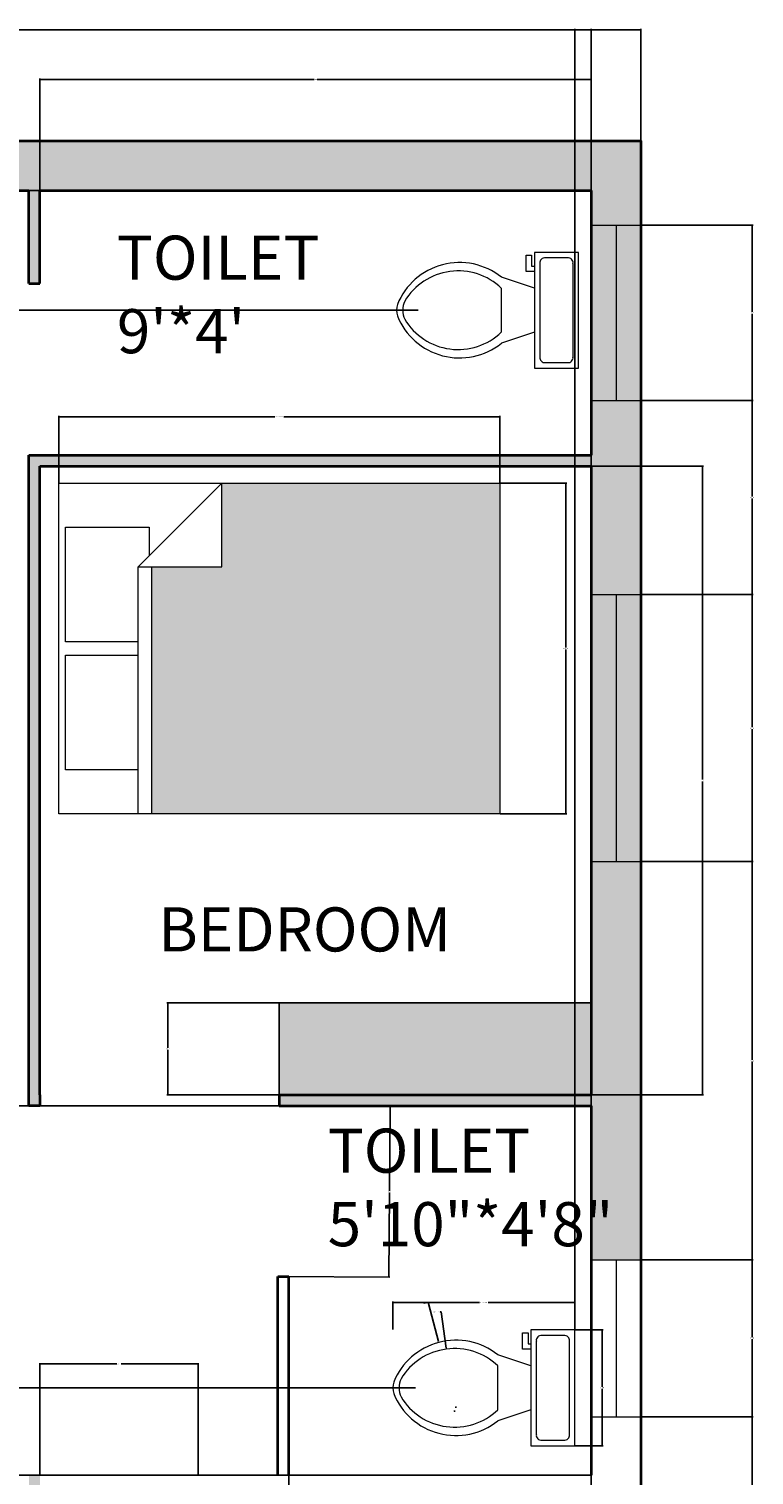
# Model space of a CAD drawing. Units: inches. Extents: x 17031430 to 17032061, y 16082759 to 16083238.
# Tile 3 of 3: x 17031585 to 17031716, y 16082898 to 16083160. Entities that reach past the tile are written whole.
import ezdxf

# ---------------------------------------------------------------- set-up
doc = ezdxf.new("R2010")
doc.units = ezdxf.units.IN
doc.header["$MEASUREMENT"] = 0
for name, color, linetype, lineweight in [('A-ANNO-DIMS', 2, 'Continuous', 18), ('A-AREA-IDEN', 7, 'Continuous', 25), ('A-FLOR-CASE', 8, 'Continuous', 25), ('A-FLOR-FIXT', 8, 'Continuous', 18), ('A-FURN', 8, 'Continuous', 18), ('A-GLAZ', 4, 'Continuous', 18), ('A-WALL', 7, 'Continuous', 35)]:
    doc.layers.add(name, color=color, linetype=linetype, lineweight=lineweight)
for name, color, linetype, lineweight, true_color in [('A-FLOR-CASE-PATT', 9, 'Continuous', 13, 0xc7c8ca), ('A-GLAZ-PATT', 252, 'Continuous', 13, 0x939598), ('A-WALL-PATT', 18, 'Continuous', 13, 0x000000)]:
    doc.layers.add(name, color=color, linetype=linetype, lineweight=lineweight, true_color=true_color)
doc.styles.get("Standard").update_dxf_attribs({"font": 'arial.ttf'})
doc.dimstyles.get("Standard").update_dxf_attribs({"dimtxt": 0.18, "dimasz": 0.18, "dimexe": 0.18, "dimexo": 0.0625, "dimgap": 0.09, "dimtad": 0, "dimtih": 1, "dimtoh": 1, "dimdec": 0, "dimzin": 0, "dimdsep": 46, "dimlunit": 3, "dimtxsty": 'Standard', "dimcen": 0.09, "dimadec": 0, "dimazin": 0, "dimtfac": 1, "dimtdec": 0, "dimtofl": 0, "dimtmove": 0, "dimatfit": 3, "dimfxl": 1, "dimtolj": 1, "dimtzin": 0, "dimarcsym": 0})

# ---------------------------------------------------------------- blocks, each defined once
blk = doc.blocks.new('Bed - Queen')
for p, q in [((0, -80.00003), (0, 0)), ((0, 0), (59.99999, 0)), ((59.99999, 0), (59.99999, -80.00003)), ((7.99999, -1.2), (28.79998, -1.2)), ((7.99999, -14.4), (7.99999, -1.2)), ((28.79998, -1.2), (28.79998, -14.4)), ((31.19999, -1.2), (51.99999, -1.2)), ((31.19999, -14.4), (31.19999, -1.2)), ((51.99999, -1.2), (51.99999, -16.4)), ((0, -14.4), (44.8, -14.4)), ((59.99999, -29.6), (44.8, -14.4)), ((44.8, -14.4), (44.8, -29.6)), ((44.8, -16.8), (0, -16.8)), ((51.99999, -16.4), (46.79936, -16.4)), ((44.8, -29.6), (59.99999, -29.6)), ((59.99999, -80.00003), (0, -80.00003))]:
    blk.add_line(p, q)
blk = doc.blocks.new('Toilet - top')
for p, q in [((9.5, -6), (9.5, -2)), ((-10, -8.5), (-8, -8.5)), ((-10, -9.5), (-10, -8.5)), ((-7, -9.5), (-10, -9.5)), ((-8, -8.5), (-8, -8)), ((-7, -8), (-7, -9.5)), ((-4, -8), (-6, -14)), ((4, -8), (6, -14)), ((4, -14), (-4, -14))]:
    blk.add_line(p, q)
blk.add_lwpolyline([(10.5, -8), (10.5, 0), (-10.5, 0), (-10.5, -8)], close=True)
for points in [[(-9.5, -2), (-9.5, -6)], [(8.5, -1), (-8.5, -1)], [(-8.5, -7), (8.5, -7)]]:
    blk.add_lwpolyline(points)
for centre, radius, start, end in [((-8.62, -1.88), 0.884, 81.8699, 188.1301), ((8.62, -1.88), 0.884, 351.8699, 98.1301), ((-8.62, -6.12), 0.884, 171.8699, 278.1301), ((8.62, -6.12), 0.884, 261.8699, 8.1301), ((3.52, -21.58), 12.17, 141.4691, 247.9714), ((4.2, -21.82), 11.33, 136.3677, 238.9468), ((-3.52, -21.58), 12.17, 292.0284, 38.5307), ((-4.2, -21.82), 11.33, 301.053, 43.6321), ((0, -27.88), 4, 245.7318, 294.2682), ((0, -29), 4, 254.8605, 285.1395)]:
    blk.add_arc(centre, radius, start, end)
blk = doc.blocks.new('*D6')
at = {"layer": 'A-ANNO-DIMS', "color": 0, "lineweight": -2, "transparency": 16777216}
for p, q in [((17031590.16, 16083077.74), (17031590.16, 16083089.86)), ((17031590.34, 16083089.68), (17031629.35, 16083089.68)), ((17031669.98, 16083089.68), (17031630.98, 16083089.68)), ((17031670.16, 16083077.74), (17031670.16, 16083089.86))]:
    blk.add_line(p, q, dxfattribs=at)
at = {"layer": 'A-ANNO-DIMS', "color": 0, "transparency": 16777216}
for points in [[(17031590.34, 16083089.71), (17031590.34, 16083089.65), (17031590.16, 16083089.68)], [(17031669.98, 16083089.71), (17031669.98, 16083089.65), (17031670.16, 16083089.68)]]:
    blk.add_solid(points, dxfattribs=at)
at = {"layer": 'Defpoints', "color": 0, "transparency": 16777216}
for p in [(17031590.16, 16083089.68), (17031590.16, 16083077.68), (17031670.16, 16083077.68)]:
    blk.add_point(p, dxfattribs=at)
at = {"layer": 'A-ANNO-DIMS', "color": 0, "transparency": 16777216, "insert": (17031630.16, 16083089.68), "char_height": 0.18, "attachment_point": 5}
blk.add_mtext('\\A1;BED 80 TYP.', dxfattribs=at)
blk = doc.blocks.new('*D7')
at = {"layer": 'A-ANNO-DIMS', "color": 0, "lineweight": -2, "transparency": 16777216}
for p, q in [((17031670.23, 16083077.68), (17031682.34, 16083077.68)), ((17031682.16, 16083077.5), (17031682.16, 16083047.86)), ((17031682.16, 16083017.86), (17031682.16, 16083047.5)), ((17031670.23, 16083017.68), (17031682.34, 16083017.68))]:
    blk.add_line(p, q, dxfattribs=at)
at = {"layer": 'A-ANNO-DIMS', "color": 0, "transparency": 16777216}
for points in [[(17031682.13, 16083077.5), (17031682.19, 16083077.5), (17031682.16, 16083077.68)], [(17031682.13, 16083017.86), (17031682.19, 16083017.86), (17031682.16, 16083017.68)]]:
    blk.add_solid(points, dxfattribs=at)
at = {"layer": 'Defpoints', "color": 0, "transparency": 16777216}
for p in [(17031670.16, 16083077.68), (17031682.16, 16083077.68), (17031670.16, 16083017.68)]:
    blk.add_point(p, dxfattribs=at)
at = {"layer": 'A-ANNO-DIMS', "color": 0, "transparency": 16777216, "insert": (17031682.16, 16083047.68), "char_height": 0.18, "attachment_point": 5}
blk.add_mtext('\\A1;60 TYP.', dxfattribs=at)
blk = doc.blocks.new('*D8')
at = {"layer": 'A-ANNO-DIMS', "color": 0, "lineweight": -2, "transparency": 16777216}
for p, q in [((17031650.74, 16082924.13), (17031650.74, 16082929.2)), ((17031650.92, 16082929.02), (17031666.49, 16082929.02)), ((17031683.6, 16082929.02), (17031668.04, 16082929.02)), ((17031683.78, 16082924.13), (17031683.78, 16082929.2))]:
    blk.add_line(p, q, dxfattribs=at)
at = {"layer": 'A-ANNO-DIMS', "color": 0, "transparency": 16777216}
for points in [[(17031650.92, 16082929.05), (17031650.92, 16082928.99), (17031650.74, 16082929.02)], [(17031683.6, 16082929.05), (17031683.6, 16082928.99), (17031683.78, 16082929.02)]]:
    blk.add_solid(points, dxfattribs=at)
at = {"layer": 'Defpoints', "color": 0, "transparency": 16777216}
for p in [(17031683.78, 16082929.02), (17031650.74, 16082924.06), (17031683.78, 16082924.06)]:
    blk.add_point(p, dxfattribs=at)
at = {"layer": 'A-ANNO-DIMS', "color": 0, "transparency": 16777216, "insert": (17031667.26, 16082929.02), "char_height": 0.18, "attachment_point": 5}
blk.add_mtext('\\A1;WC 33 TYP.', dxfattribs=at)
blk = doc.blocks.new('*D9')
at = {"layer": 'A-ANNO-DIMS', "color": 0, "lineweight": -2, "transparency": 16777216}
for p, q in [((17031683.85, 16082924.06), (17031688.92, 16082924.06)), ((17031688.74, 16082923.88), (17031688.74, 16082913.74)), ((17031688.74, 16082903.24), (17031688.74, 16082913.38)), ((17031683.85, 16082903.06), (17031688.92, 16082903.06))]:
    blk.add_line(p, q, dxfattribs=at)
at = {"layer": 'A-ANNO-DIMS', "color": 0, "transparency": 16777216}
for points in [[(17031688.71, 16082923.88), (17031688.77, 16082923.88), (17031688.74, 16082924.06)], [(17031688.71, 16082903.24), (17031688.77, 16082903.24), (17031688.74, 16082903.06)]]:
    blk.add_solid(points, dxfattribs=at)
at = {"layer": 'Defpoints', "color": 0, "transparency": 16777216}
for p in [(17031683.78, 16082924.06), (17031683.78, 16082903.06), (17031688.74, 16082903.06)]:
    blk.add_point(p, dxfattribs=at)
at = {"layer": 'A-ANNO-DIMS', "color": 0, "transparency": 16777216, "insert": (17031688.74, 16082913.56), "char_height": 0.18, "attachment_point": 5}
blk.add_mtext('\\A1;21 TYP.', dxfattribs=at)
blk = doc.blocks.new('*D14')
at = {"layer": 'A-ANNO-DIMS', "color": 0, "lineweight": -2, "transparency": 16777216}
for p, q in [((17031455.76, 16083139.8), (17031455.76, 16083160.07)), ((17031455.94, 16083159.89), (17031575.47, 16083159.89)), ((17031695.58, 16083159.89), (17031576.05, 16083159.89)), ((17031695.76, 16083139.8), (17031695.76, 16083160.07))]:
    blk.add_line(p, q, dxfattribs=at)
at = {"layer": 'A-ANNO-DIMS', "color": 0, "transparency": 16777216}
for points in [[(17031455.94, 16083159.92), (17031455.94, 16083159.86), (17031455.76, 16083159.89)], [(17031695.58, 16083159.92), (17031695.58, 16083159.86), (17031695.76, 16083159.89)]]:
    blk.add_solid(points, dxfattribs=at)
at = {"layer": 'Defpoints', "color": 0, "transparency": 16777216}
for p in [(17031695.76, 16083159.89), (17031455.76, 16083139.74), (17031695.76, 16083139.74)]:
    blk.add_point(p, dxfattribs=at)
at = {"layer": 'A-ANNO-DIMS', "color": 0, "transparency": 16777216, "insert": (17031575.76, 16083159.89), "char_height": 0.18, "attachment_point": 5}
blk.add_mtext('\\A1;240', dxfattribs=at)
blk = doc.blocks.new('*D18')
at = {"layer": 'A-ANNO-DIMS', "color": 0, "lineweight": -2, "transparency": 16777216}
for p, q in [((17031586.76, 16083130.8), (17031586.76, 16083151.07)), ((17031586.94, 16083150.89), (17031636.48, 16083150.89)), ((17031686.58, 16083150.89), (17031637.04, 16083150.89)), ((17031686.76, 16083130.8), (17031686.76, 16083151.07))]:
    blk.add_line(p, q, dxfattribs=at)
at = {"layer": 'A-ANNO-DIMS', "color": 0, "transparency": 16777216}
for points in [[(17031586.94, 16083150.92), (17031586.94, 16083150.86), (17031586.76, 16083150.89)], [(17031686.58, 16083150.92), (17031686.58, 16083150.86), (17031686.76, 16083150.89)]]:
    blk.add_solid(points, dxfattribs=at)
at = {"layer": 'Defpoints', "color": 0, "transparency": 16777216}
for p in [(17031686.76, 16083150.89), (17031586.76, 16083130.74), (17031686.76, 16083130.74)]:
    blk.add_point(p, dxfattribs=at)
at = {"layer": 'A-ANNO-DIMS', "color": 0, "transparency": 16777216, "insert": (17031636.76, 16083150.89), "char_height": 0.18, "attachment_point": 5}
blk.add_mtext('\\A1;100', dxfattribs=at)
blk = doc.blocks.new('*D27')
at = {"layer": 'A-ANNO-DIMS', "color": 0, "lineweight": -2, "transparency": 16777216}
for p, q in [((17031695.82, 16082908.33), (17031716.09, 16082908.33)), ((17031715.91, 16082908.15), (17031715.91, 16082844.22)), ((17031715.91, 16082779.92), (17031715.91, 16082843.85)), ((17031695.82, 16082779.74), (17031716.09, 16082779.74))]:
    blk.add_line(p, q, dxfattribs=at)
at = {"layer": 'A-ANNO-DIMS', "color": 0, "transparency": 16777216}
for points in [[(17031715.88, 16082908.15), (17031715.94, 16082908.15), (17031715.91, 16082908.33)], [(17031715.88, 16082779.92), (17031715.94, 16082779.92), (17031715.91, 16082779.74)]]:
    blk.add_solid(points, dxfattribs=at)
at = {"layer": 'Defpoints', "color": 0, "transparency": 16777216}
for p in [(17031695.76, 16082908.33), (17031695.76, 16082779.74), (17031715.91, 16082779.74)]:
    blk.add_point(p, dxfattribs=at)
at = {"layer": 'A-ANNO-DIMS', "color": 0, "transparency": 16777216, "insert": (17031715.91, 16082844.04), "char_height": 0.18, "attachment_point": 5}
blk.add_mtext('\\A1;128.6', dxfattribs=at)
blk = doc.blocks.new('*D28')
at = {"layer": 'A-ANNO-DIMS', "color": 0, "lineweight": -2, "transparency": 16777216}
for p, q in [((17031695.82, 16082936.79), (17031716.09, 16082936.79)), ((17031715.91, 16082936.61), (17031715.91, 16082922.74)), ((17031715.91, 16082908.51), (17031715.91, 16082922.38)), ((17031695.82, 16082908.33), (17031716.09, 16082908.33))]:
    blk.add_line(p, q, dxfattribs=at)
at = {"layer": 'A-ANNO-DIMS', "color": 0, "transparency": 16777216}
for points in [[(17031715.88, 16082936.61), (17031715.94, 16082936.61), (17031715.91, 16082936.79)], [(17031715.88, 16082908.51), (17031715.94, 16082908.51), (17031715.91, 16082908.33)]]:
    blk.add_solid(points, dxfattribs=at)
at = {"layer": 'Defpoints', "color": 0, "transparency": 16777216}
for p in [(17031695.76, 16082936.79), (17031715.91, 16082936.79), (17031695.76, 16082908.33)]:
    blk.add_point(p, dxfattribs=at)
at = {"layer": 'A-ANNO-DIMS', "color": 0, "transparency": 16777216, "insert": (17031715.91, 16082922.56), "char_height": 0.18, "attachment_point": 5}
blk.add_mtext('\\A1;28.455', dxfattribs=at)
blk = doc.blocks.new('*D29')
at = {"layer": 'A-ANNO-DIMS', "color": 0, "lineweight": -2, "transparency": 16777216}
for p, q in [((17031695.82, 16083009.02), (17031716.09, 16083009.02)), ((17031715.91, 16083008.84), (17031715.91, 16082973.08)), ((17031715.91, 16082936.97), (17031715.91, 16082972.72)), ((17031695.82, 16082936.79), (17031716.09, 16082936.79))]:
    blk.add_line(p, q, dxfattribs=at)
at = {"layer": 'A-ANNO-DIMS', "color": 0, "transparency": 16777216}
for points in [[(17031715.88, 16083008.84), (17031715.94, 16083008.84), (17031715.91, 16083009.02)], [(17031715.88, 16082936.97), (17031715.94, 16082936.97), (17031715.91, 16082936.79)]]:
    blk.add_solid(points, dxfattribs=at)
at = {"layer": 'Defpoints', "color": 0, "transparency": 16777216}
for p in [(17031695.76, 16083009.02), (17031695.76, 16082936.79), (17031715.91, 16082936.79)]:
    blk.add_point(p, dxfattribs=at)
at = {"layer": 'A-ANNO-DIMS', "color": 0, "transparency": 16777216, "insert": (17031715.91, 16082972.9), "char_height": 0.18, "attachment_point": 5}
blk.add_mtext('\\A1;72.23', dxfattribs=at)
blk = doc.blocks.new('*D30')
at = {"layer": 'A-ANNO-DIMS', "color": 0, "lineweight": -2, "transparency": 16777216}
for p, q in [((17031695.82, 16083057.47), (17031716.09, 16083057.47)), ((17031715.91, 16083057.29), (17031715.91, 16083033.42)), ((17031715.91, 16083009.2), (17031715.91, 16083033.06)), ((17031695.82, 16083009.02), (17031716.09, 16083009.02))]:
    blk.add_line(p, q, dxfattribs=at)
at = {"layer": 'A-ANNO-DIMS', "color": 0, "transparency": 16777216}
for points in [[(17031715.88, 16083057.29), (17031715.94, 16083057.29), (17031715.91, 16083057.47)], [(17031715.88, 16083009.2), (17031715.94, 16083009.2), (17031715.91, 16083009.02)]]:
    blk.add_solid(points, dxfattribs=at)
at = {"layer": 'Defpoints', "color": 0, "transparency": 16777216}
for p in [(17031695.76, 16083057.47), (17031695.76, 16083009.02), (17031715.91, 16083009.02)]:
    blk.add_point(p, dxfattribs=at)
at = {"layer": 'A-ANNO-DIMS', "color": 0, "transparency": 16777216, "insert": (17031715.91, 16083033.24), "char_height": 0.18, "attachment_point": 5}
blk.add_mtext('\\A1;48.45', dxfattribs=at)
blk = doc.blocks.new('*D31')
at = {"layer": 'A-ANNO-DIMS', "color": 0, "lineweight": -2, "transparency": 16777216}
for p, q in [((17031695.82, 16083092.69), (17031716.09, 16083092.69)), ((17031715.91, 16083092.51), (17031715.91, 16083075.26)), ((17031715.91, 16083057.65), (17031715.91, 16083074.9)), ((17031695.82, 16083057.47), (17031716.09, 16083057.47))]:
    blk.add_line(p, q, dxfattribs=at)
at = {"layer": 'A-ANNO-DIMS', "color": 0, "transparency": 16777216}
for points in [[(17031715.88, 16083092.51), (17031715.94, 16083092.51), (17031715.91, 16083092.69)], [(17031715.88, 16083057.65), (17031715.94, 16083057.65), (17031715.91, 16083057.47)]]:
    blk.add_solid(points, dxfattribs=at)
at = {"layer": 'Defpoints', "color": 0, "transparency": 16777216}
for p in [(17031695.76, 16083092.69), (17031695.76, 16083057.47), (17031715.91, 16083057.47)]:
    blk.add_point(p, dxfattribs=at)
at = {"layer": 'A-ANNO-DIMS', "color": 0, "transparency": 16777216, "insert": (17031715.91, 16083075.08), "char_height": 0.18, "attachment_point": 5}
blk.add_mtext('\\A1;35.23', dxfattribs=at)
blk = doc.blocks.new('*D32')
at = {"layer": 'A-ANNO-DIMS', "color": 0, "lineweight": -2, "transparency": 16777216}
for p, q in [((17031695.82, 16083124.5), (17031716.09, 16083124.5)), ((17031715.91, 16083124.32), (17031715.91, 16083108.78)), ((17031715.91, 16083092.87), (17031715.91, 16083108.41)), ((17031695.82, 16083092.69), (17031716.09, 16083092.69))]:
    blk.add_line(p, q, dxfattribs=at)
at = {"layer": 'A-ANNO-DIMS', "color": 0, "transparency": 16777216}
for points in [[(17031715.88, 16083124.32), (17031715.94, 16083124.32), (17031715.91, 16083124.5)], [(17031715.88, 16083092.87), (17031715.94, 16083092.87), (17031715.91, 16083092.69)]]:
    blk.add_solid(points, dxfattribs=at)
at = {"layer": 'Defpoints', "color": 0, "transparency": 16777216}
for p in [(17031695.76, 16083124.5), (17031695.76, 16083092.69), (17031715.91, 16083092.69)]:
    blk.add_point(p, dxfattribs=at)
at = {"layer": 'A-ANNO-DIMS', "color": 0, "transparency": 16777216, "insert": (17031715.91, 16083108.6), "char_height": 0.18, "attachment_point": 5}
blk.add_mtext('\\A1;31.8', dxfattribs=at)
blk = doc.blocks.new('*D37')
at = {"layer": 'A-ANNO-DIMS', "color": 0, "lineweight": -2, "transparency": 16777216}
for p, q in [((17031686.82, 16083080.74), (17031707.09, 16083080.74)), ((17031706.91, 16083080.56), (17031706.91, 16083023.92)), ((17031706.91, 16082966.92), (17031706.91, 16083023.56)), ((17031686.82, 16082966.74), (17031707.09, 16082966.74))]:
    blk.add_line(p, q, dxfattribs=at)
at = {"layer": 'A-ANNO-DIMS', "color": 0, "transparency": 16777216}
for points in [[(17031706.88, 16083080.56), (17031706.94, 16083080.56), (17031706.91, 16083080.74)], [(17031706.88, 16082966.92), (17031706.94, 16082966.92), (17031706.91, 16082966.74)]]:
    blk.add_solid(points, dxfattribs=at)
at = {"layer": 'Defpoints', "color": 0, "transparency": 16777216}
for p in [(17031686.76, 16083080.74), (17031686.76, 16082966.74), (17031706.91, 16082966.74)]:
    blk.add_point(p, dxfattribs=at)
at = {"layer": 'A-ANNO-DIMS', "color": 0, "transparency": 16777216, "insert": (17031706.91, 16083023.74), "char_height": 0.18, "attachment_point": 5}
blk.add_mtext('\\A1;114', dxfattribs=at)
blk = doc.blocks.new('*D40')
at = {"layer": 'A-ANNO-DIMS', "color": 0, "lineweight": -2, "transparency": 16777216}
for p, q in [((17031586.76, 16082897.8), (17031586.76, 16082918.07)), ((17031586.94, 16082917.89), (17031600.73, 16082917.89)), ((17031615.28, 16082917.89), (17031601.49, 16082917.89)), ((17031615.46, 16082897.8), (17031615.46, 16082918.07))]:
    blk.add_line(p, q, dxfattribs=at)
at = {"layer": 'A-ANNO-DIMS', "color": 0, "transparency": 16777216}
for points in [[(17031586.94, 16082917.92), (17031586.94, 16082917.86), (17031586.76, 16082917.89)], [(17031615.28, 16082917.92), (17031615.28, 16082917.86), (17031615.46, 16082917.89)]]:
    blk.add_solid(points, dxfattribs=at)
at = {"layer": 'Defpoints', "color": 0, "transparency": 16777216}
for p in [(17031615.46, 16082917.89), (17031586.76, 16082897.74), (17031615.46, 16082897.74)]:
    blk.add_point(p, dxfattribs=at)
at = {"layer": 'A-ANNO-DIMS', "color": 0, "transparency": 16777216, "insert": (17031601.11, 16082917.89), "char_height": 0.18, "attachment_point": 5}
blk.add_mtext('\\A1;28.71', dxfattribs=at)
blk = doc.blocks.new('*D42')
at = {"layer": 'A-ANNO-DIMS', "color": 0, "lineweight": -2, "transparency": 16777216}
for p, q in [((17031630.18, 16082964.74), (17031650.45, 16082964.6)), ((17031650.27, 16082964.43), (17031650.17, 16082949.31)), ((17031650.06, 16082933.84), (17031650.17, 16082948.95)), ((17031629.98, 16082933.79), (17031650.24, 16082933.65))]:
    blk.add_line(p, q, dxfattribs=at)
at = {"layer": 'A-ANNO-DIMS', "color": 0, "transparency": 16777216}
for points in [[(17031650.24, 16082964.43), (17031650.3, 16082964.43), (17031650.27, 16082964.61)], [(17031650.03, 16082933.84), (17031650.09, 16082933.84), (17031650.06, 16082933.66)]]:
    blk.add_solid(points, dxfattribs=at)
at = {"layer": 'Defpoints', "color": 0, "transparency": 16777216}
for p in [(17031630.12, 16082964.74), (17031629.91, 16082933.79), (17031650.06, 16082933.66)]:
    blk.add_point(p, dxfattribs=at)
at = {"layer": 'A-ANNO-DIMS', "color": 0, "transparency": 16777216, "insert": (17031650.17, 16082949.13), "char_height": 0.18, "attachment_point": 5}
blk.add_mtext('\\A1;30.95', dxfattribs=at)
blk = doc.blocks.new('*D43')
at = {"layer": 'A-ANNO-DIMS', "color": 0, "lineweight": -2, "transparency": 16777216}
for p, q in [((17031631.91, 16082897.68), (17031631.91, 16082759.41)), ((17031686.76, 16082897.68), (17031686.76, 16082759.41)), ((17031632.09, 16082759.59), (17031658.94, 16082759.59)), ((17031686.58, 16082759.59), (17031659.73, 16082759.59))]:
    blk.add_line(p, q, dxfattribs=at)
at = {"layer": 'A-ANNO-DIMS', "color": 0, "transparency": 16777216}
for points in [[(17031632.09, 16082759.62), (17031632.09, 16082759.56), (17031631.91, 16082759.59)], [(17031686.58, 16082759.62), (17031686.58, 16082759.56), (17031686.76, 16082759.59)]]:
    blk.add_solid(points, dxfattribs=at)
at = {"layer": 'Defpoints', "color": 0, "transparency": 16777216}
for p in [(17031631.91, 16082897.74), (17031686.76, 16082897.74), (17031686.76, 16082759.59)]:
    blk.add_point(p, dxfattribs=at)
at = {"layer": 'A-ANNO-DIMS', "color": 0, "transparency": 16777216, "insert": (17031659.34, 16082759.59), "char_height": 0.18, "attachment_point": 5}
blk.add_mtext('\\A1;54.84', dxfattribs=at)
blk = doc.blocks.new('*D44')
at = {"layer": 'A-ANNO-DIMS', "color": 0, "lineweight": -2, "transparency": 16777216}
for p, q in [((17031630.06, 16082964.74), (17031435.43, 16082964.74)), ((17031435.61, 16082964.56), (17031435.61, 16082931.42)), ((17031435.61, 16082897.92), (17031435.61, 16082931.06)), ((17031629.85, 16082897.74), (17031435.43, 16082897.74))]:
    blk.add_line(p, q, dxfattribs=at)
at = {"layer": 'A-ANNO-DIMS', "color": 0, "transparency": 16777216}
for points in [[(17031435.58, 16082964.56), (17031435.64, 16082964.56), (17031435.61, 16082964.74)], [(17031435.58, 16082897.92), (17031435.64, 16082897.92), (17031435.61, 16082897.74)]]:
    blk.add_solid(points, dxfattribs=at)
at = {"layer": 'Defpoints', "color": 0, "transparency": 16777216}
for p in [(17031435.61, 16082964.74), (17031630.12, 16082964.74), (17031629.91, 16082897.74)]:
    blk.add_point(p, dxfattribs=at)
at = {"layer": 'A-ANNO-DIMS', "color": 0, "transparency": 16777216, "insert": (17031435.61, 16082931.24), "char_height": 0.18, "attachment_point": 5}
blk.add_mtext('\\A1;67', dxfattribs=at)
blk = doc.blocks.new('*D52')
at = {"layer": 'A-ANNO-DIMS', "color": 0, "lineweight": -2, "transparency": 16777216}
for p, q in [((17031630.06, 16082983.39), (17031609.79, 16082983.39)), ((17031609.97, 16082983.21), (17031609.97, 16082975.25)), ((17031609.97, 16082966.92), (17031609.97, 16082974.88)), ((17031630.06, 16082966.74), (17031609.79, 16082966.74))]:
    blk.add_line(p, q, dxfattribs=at)
at = {"layer": 'A-ANNO-DIMS', "color": 0, "transparency": 16777216}
for points in [[(17031609.94, 16082983.21), (17031610, 16082983.21), (17031609.97, 16082983.39)], [(17031609.94, 16082966.92), (17031610, 16082966.92), (17031609.97, 16082966.74)]]:
    blk.add_solid(points, dxfattribs=at)
at = {"layer": 'Defpoints', "color": 0, "transparency": 16777216}
for p in [(17031609.97, 16082983.39), (17031630.12, 16082983.39), (17031630.12, 16082966.74)]:
    blk.add_point(p, dxfattribs=at)
at = {"layer": 'A-ANNO-DIMS', "color": 0, "transparency": 16777216, "insert": (17031609.97, 16082975.06), "char_height": 0.18, "attachment_point": 5}
blk.add_mtext('\\A1;16.647', dxfattribs=at)
blk = doc.blocks.new('*D53')
at = {"layer": 'A-ANNO-DIMS', "color": 0, "lineweight": -2, "transparency": 16777216}
for p, q in [((17031654.72, 16082913.56), (17031435.43, 16082913.56)), ((17031435.61, 16082913.38), (17031435.61, 16082905.83)), ((17031435.61, 16082897.92), (17031435.61, 16082905.47)), ((17031686.69, 16082897.74), (17031435.43, 16082897.74))]:
    blk.add_line(p, q, dxfattribs=at)
at = {"layer": 'A-ANNO-DIMS', "color": 0, "transparency": 16777216}
for points in [[(17031435.58, 16082913.38), (17031435.64, 16082913.38), (17031435.61, 16082913.56)], [(17031435.58, 16082897.92), (17031435.64, 16082897.92), (17031435.61, 16082897.74)]]:
    blk.add_solid(points, dxfattribs=at)
at = {"layer": 'Defpoints', "color": 0, "transparency": 16777216}
for p in [(17031435.61, 16082913.56), (17031654.78, 16082913.56), (17031686.76, 16082897.74)]:
    blk.add_point(p, dxfattribs=at)
at = {"layer": 'A-ANNO-DIMS', "color": 0, "transparency": 16777216, "insert": (17031435.61, 16082905.65), "char_height": 0.18, "attachment_point": 5}
blk.add_mtext('\\A1;15.824', dxfattribs=at)
blk = doc.blocks.new('*D54')
at = {"layer": 'A-ANNO-DIMS', "color": 0, "lineweight": -2, "transparency": 16777216}
for p, q in [((17031683.78, 16082924.13), (17031683.78, 16083160.07)), ((17031683.96, 16083159.89), (17031684.95, 16083159.89)), ((17031686.58, 16083159.89), (17031685.6, 16083159.89)), ((17031686.76, 16082936.85), (17031686.76, 16083160.07))]:
    blk.add_line(p, q, dxfattribs=at)
at = {"layer": 'A-ANNO-DIMS', "color": 0, "transparency": 16777216}
for points in [[(17031683.96, 16083159.92), (17031683.96, 16083159.86), (17031683.78, 16083159.89)], [(17031686.58, 16083159.92), (17031686.58, 16083159.86), (17031686.76, 16083159.89)]]:
    blk.add_solid(points, dxfattribs=at)
at = {"layer": 'Defpoints', "color": 0, "transparency": 16777216}
for p in [(17031686.76, 16083159.89), (17031686.76, 16082936.79), (17031683.78, 16082924.06)]:
    blk.add_point(p, dxfattribs=at)
at = {"layer": 'A-ANNO-DIMS', "color": 0, "transparency": 16777216, "insert": (17031685.27, 16083159.89), "char_height": 0.18, "attachment_point": 5}
blk.add_mtext('\\A1;2.97', dxfattribs=at)
blk = doc.blocks.new('*D55')
at = {"layer": 'A-ANNO-DIMS', "color": 0, "lineweight": -2, "transparency": 16777216}
for p, q in [((17031686.69, 16083130.74), (17031435.43, 16083130.74)), ((17031435.61, 16083130.56), (17031435.61, 16083120.07)), ((17031435.61, 16083109.22), (17031435.61, 16083119.71)), ((17031655.38, 16083109.04), (17031435.43, 16083109.04))]:
    blk.add_line(p, q, dxfattribs=at)
at = {"layer": 'A-ANNO-DIMS', "color": 0, "transparency": 16777216}
for points in [[(17031435.58, 16083130.56), (17031435.64, 16083130.56), (17031435.61, 16083130.74)], [(17031435.58, 16083109.22), (17031435.64, 16083109.22), (17031435.61, 16083109.04)]]:
    blk.add_solid(points, dxfattribs=at)
at = {"layer": 'Defpoints', "color": 0, "transparency": 16777216}
for p in [(17031686.76, 16083130.74), (17031435.61, 16083109.04), (17031655.44, 16083109.04)]:
    blk.add_point(p, dxfattribs=at)
at = {"layer": 'A-ANNO-DIMS', "color": 0, "transparency": 16777216, "insert": (17031435.61, 16083119.89), "char_height": 0.18, "attachment_point": 5}
blk.add_mtext('\\A1;21.7', dxfattribs=at)
blk = doc.blocks.new('*D58')
at = {"layer": 'A-ANNO-DIMS', "color": 0, "lineweight": -2, "transparency": 16777216}
for p, q in [((17031657.08, 16082928.88), (17031657.26, 16082928.88)), ((17031657.26, 16082928.88), (17031659.07, 16082921.99)), ((17031662.11, 16082910.04), (17031662.29, 16082910.04)), ((17031662.2, 16082909.95), (17031662.2, 16082910.13))]:
    blk.add_line(p, q, dxfattribs=at)
at = {"layer": 'A-ANNO-DIMS', "color": 0, "transparency": 16777216}
blk.add_solid([(17031659.1, 16082922), (17031659.04, 16082921.98), (17031659.11, 16082921.81)], dxfattribs=at)
at = {"layer": 'Defpoints', "color": 0, "transparency": 16777216}
for p in [(17031659.11, 16082921.81), (17031662.2, 16082910.04)]:
    blk.add_point(p, dxfattribs=at)
at = {"layer": 'A-ANNO-DIMS', "color": 0, "transparency": 16777216, "insert": (17031656.4, 16082928.88), "char_height": 0.18, "attachment_point": 5}
blk.add_mtext('\\A1;4X R12.17', dxfattribs=at)
blk = doc.blocks.new('*D59')
at = {"layer": 'A-ANNO-DIMS', "color": 0, "lineweight": -2, "transparency": 16777216}
for p, q in [((17031659.37, 16082927.33), (17031659.55, 16082927.33)), ((17031659.55, 16082927.33), (17031660.43, 16082920.77)), ((17031661.88, 16082909.36), (17031662.06, 16082909.36)), ((17031661.97, 16082909.27), (17031661.97, 16082909.45))]:
    blk.add_line(p, q, dxfattribs=at)
at = {"layer": 'A-ANNO-DIMS', "color": 0, "transparency": 16777216}
blk.add_solid([(17031660.46, 16082920.77), (17031660.4, 16082920.77), (17031660.46, 16082920.59)], dxfattribs=at)
at = {"layer": 'Defpoints', "color": 0, "transparency": 16777216}
for p in [(17031660.46, 16082920.59), (17031661.97, 16082909.36)]:
    blk.add_point(p, dxfattribs=at)
at = {"layer": 'A-ANNO-DIMS', "color": 0, "transparency": 16777216, "insert": (17031658.7, 16082927.33), "char_height": 0.18, "attachment_point": 5}
blk.add_mtext('\\A1;4X R11.33', dxfattribs=at)
blk = doc.blocks.new('*D60')
at = {"layer": 'A-ANNO-DIMS', "color": 0, "lineweight": -2, "transparency": 16777216}
for p, q in [((17031648.38, 16082913.56), (17031650.6, 16082913.56)), ((17031654.69, 16082913.56), (17031654.87, 16082913.56)), ((17031654.78, 16082913.47), (17031654.78, 16082913.65))]:
    blk.add_line(p, q, dxfattribs=at)
at = {"layer": 'A-ANNO-DIMS', "color": 0, "transparency": 16777216}
blk.add_solid([(17031650.6, 16082913.59), (17031650.6, 16082913.53), (17031650.78, 16082913.56)], dxfattribs=at)
at = {"layer": 'Defpoints', "color": 0, "transparency": 16777216}
for p in [(17031650.78, 16082913.56), (17031654.78, 16082913.56)]:
    blk.add_point(p, dxfattribs=at)
at = {"layer": 'A-ANNO-DIMS', "color": 0, "transparency": 16777216, "insert": (17031647.95, 16082913.56), "char_height": 0.18, "attachment_point": 5}
blk.add_mtext('\\A1;4X R4', dxfattribs=at)

msp = doc.modelspace()

# ---------------------------------------------------------------- hatches: boundary and pattern name
at = {"layer": 'A-FLOR-CASE-PATT'}
h = msp.add_hatch(dxfattribs=at)
h.set_pattern_fill('ANSI38', color=256, scale=1.5)
h.set_pattern_definition([(45, (0, 0), (-0.1325825214725, 0.1325825214725), []), (135, (0, 0), (-0.3977475644174, 0.1325825214725), [0.46875, -0.28125])])
h.paths.add_polyline_path([(17031686.7571, 16082983.3874), (17031630.1205, 16082983.3874), (17031630.1205, 16082966.7405), (17031686.7571, 16082966.7405)])
at = {"layer": 'A-GLAZ-PATT'}
h = msp.add_hatch(color=256, dxfattribs=at)
h.dxf.hatch_style = 1
h.paths.add_polyline_path([(17031546.2248, 16083139.7405), (17031495.2896, 16083139.7405), (17031495.2896, 16083135.2405), (17031546.2248, 16083135.2405)])
h.paths.add_polyline_path([(17031546.2248, 16083135.2405), (17031495.2896, 16083135.2405), (17031495.2896, 16083130.7405), (17031546.2248, 16083130.7405)])
h.paths.add_polyline_path([(17031464.7571, 16083099.8263), (17031460.2571, 16083099.8263), (17031460.2571, 16083058.1685), (17031464.7571, 16083058.1685)])
h.paths.add_polyline_path([(17031460.2571, 16083099.8263), (17031455.7571, 16083099.8263), (17031455.7571, 16083058.1685), (17031460.2571, 16083058.1685)])
h.paths.add_polyline_path([(17031464.7571, 16082953.9805), (17031460.2571, 16082953.9805), (17031460.2571, 16082911.6971), (17031464.7571, 16082911.6971)])
h.paths.add_polyline_path([(17031460.2571, 16082953.9805), (17031455.7571, 16082953.9805), (17031455.7571, 16082911.6971), (17031460.2571, 16082911.6971)])
h.paths.add_polyline_path([(17031460.2571, 16082862.954), (17031455.7571, 16082862.954), (17031455.7571, 16082807.1802), (17031460.2571, 16082807.1802)])
h.paths.add_polyline_path([(17031464.7571, 16082862.954), (17031460.2571, 16082862.954), (17031460.2571, 16082807.1802), (17031464.7571, 16082807.1802)])
h.paths.add_polyline_path([(17031681.0952, 16082784.2405), (17031647.5287, 16082784.2405), (17031647.5287, 16082779.7405), (17031681.0952, 16082779.7405)])
h.paths.add_polyline_path([(17031681.0952, 16082788.7405), (17031647.5287, 16082788.7405), (17031647.5287, 16082784.2405), (17031681.0952, 16082784.2405)])
h.paths.add_polyline_path([(17031691.2571, 16083057.4652), (17031686.7571, 16083057.4652), (17031686.7571, 16083009.0162), (17031691.2571, 16083009.0162)])
h.paths.add_polyline_path([(17031514.2108, 16082846.7675), (17031567.264, 16082846.7675), (17031567.264, 16082876.6193), (17031514.2108, 16082876.6193)], flags=9)
h.paths.add_polyline_path([(17031636.4861, 16082934.711), (17031688.115, 16082934.711), (17031688.115, 16082964.5628), (17031636.4861, 16082964.5628)], flags=9)
h.paths.add_polyline_path([(17031509.9735, 16082952.8397), (17031561.3568, 16082952.8397), (17031561.3568, 16082996.1612), (17031509.9735, 16082996.1612)], flags=9)
h.paths.add_polyline_path([(17031605.4082, 16082988.2134), (17031667.1545, 16082988.2134), (17031667.1545, 16083004.6991), (17031605.4082, 16083004.6991)], flags=9)
h.paths.add_polyline_path([(17031598.2513, 16083096.6971), (17031641.5746, 16083096.6971), (17031641.5746, 16083126.5489), (17031598.2513, 16083126.5489)], flags=9)
h.paths.add_polyline_path([(17031536.0858, 16083028.4916), (17031577.5319, 16083028.4916), (17031577.5319, 16083058.3434), (17031536.0858, 16083058.3434)], flags=9)
h = msp.add_hatch(color=256, dxfattribs=at)
h.dxf.hatch_style = 1
h.paths.add_polyline_path([(17031695.7571, 16083124.4975), (17031691.2571, 16083124.4975), (17031691.2571, 16083092.6946), (17031695.7571, 16083092.6946)])
h.paths.add_polyline_path([(17031691.2571, 16083124.4975), (17031686.7571, 16083124.4975), (17031686.7571, 16083092.6946), (17031691.2571, 16083092.6946)])
h.paths.add_polyline_path([(17031695.7571, 16083057.4652), (17031691.2571, 16083057.4652), (17031691.2571, 16083009.0162), (17031695.7571, 16083009.0162)])
h.paths.add_polyline_path([(17031534.8905, 16083097.4163), (17031519.6905, 16083097.4163), (17031519.6905, 16083110.2163), (17031474.8905, 16083110.2163), (17031474.8905, 16083047.0163), (17031534.8905, 16083047.0163)])
h.paths.add_polyline_path([(17031670.1648, 16083077.6823), (17031619.7648, 16083077.6823), (17031619.7648, 16083062.4823), (17031606.9648, 16083062.4823), (17031606.9648, 16083017.6823), (17031670.1648, 16083017.6823)])
at = {"layer": 'A-WALL-PATT'}
h = msp.add_hatch(color=256, dxfattribs=at)
h.dxf.hatch_style = 1
h.paths.add_polyline_path([(17031695.7571, 16083009.0162), (17031686.7571, 16083009.0162), (17031686.7571, 16082966.7405), (17031630.1205, 16082966.7405), (17031630.1205, 16082964.7405), (17031686.7571, 16082964.7405), (17031686.7571, 16082936.7854), (17031695.7571, 16082936.7854)])
h.paths.add_polyline_path([(17031695.7571, 16083092.6946), (17031686.7571, 16083092.6946), (17031686.7571, 16083082.7405), (17031584.7571, 16083082.7405), (17031584.7571, 16083019.7405), (17031584.7571, 16083017.7405), (17031584.7571, 16082966.7405), (17031584.7571, 16082964.7405), (17031586.7571, 16082964.7405), (17031586.7571, 16082966.7405), (17031586.7571, 16083080.7405), (17031686.7571, 16083080.7405), (17031686.7571, 16083057.4652), (17031695.7571, 16083057.4652)])
h.paths.add_polyline_path([(17031695.7571, 16083139.7405), (17031546.2248, 16083139.7405), (17031546.2248, 16083130.7405), (17031584.7571, 16083130.7405), (17031584.7571, 16083113.9162), (17031586.7571, 16083113.9162), (17031586.7571, 16083130.7405), (17031686.7571, 16083130.7405), (17031686.7571, 16083124.4975), (17031695.7571, 16083124.4975)])
h.paths.add_polyline_path([(17031495.2896, 16083139.7405), (17031455.7571, 16083139.7405), (17031455.7571, 16083099.8263), (17031464.7571, 16083099.8263), (17031464.7571, 16083130.7405), (17031495.2896, 16083130.7405)])
h.paths.add_polyline_path([(17031537.499, 16083019.7405), (17031464.7571, 16083019.7405), (17031464.7571, 16083058.1685), (17031455.7571, 16083058.1685), (17031455.7571, 16082953.9805), (17031464.7571, 16082953.9805), (17031464.7571, 16083017.7405), (17031537.499, 16083017.7405)])
h.paths.add_polyline_path([(17031464.7571, 16082911.6971), (17031455.7571, 16082911.6971), (17031455.7571, 16082862.954), (17031464.7571, 16082862.954), (17031464.7571, 16082895.7405), (17031548.467, 16082895.7405), (17031548.467, 16082897.7405), (17031464.7571, 16082897.7405)])
h.paths.add_polyline_path([(17031464.7571, 16082807.1802), (17031455.7571, 16082807.1802), (17031455.7571, 16082779.7405), (17031647.5287, 16082779.7405), (17031647.5287, 16082788.7405), (17031586.7571, 16082788.7405), (17031586.7571, 16082897.7405), (17031584.7571, 16082897.7405), (17031584.7571, 16082895.7405), (17031584.7571, 16082788.7405), (17031464.7571, 16082788.7405)])
h.paths.add_polyline_path([(17031514.2108, 16082846.7675), (17031567.264, 16082846.7675), (17031567.264, 16082876.6193), (17031514.2108, 16082876.6193)], flags=25)
h.paths.add_polyline_path([(17031636.4861, 16082934.711), (17031688.115, 16082934.711), (17031688.115, 16082964.5628), (17031636.4861, 16082964.5628)], flags=9)
h.paths.add_polyline_path([(17031509.9735, 16082952.8397), (17031561.3568, 16082952.8397), (17031561.3568, 16082996.1612), (17031509.9735, 16082996.1612)], flags=9)
h.paths.add_polyline_path([(17031605.4082, 16082988.2134), (17031667.1545, 16082988.2134), (17031667.1545, 16083004.6991), (17031605.4082, 16083004.6991)], flags=25)
h.paths.add_polyline_path([(17031598.2513, 16083096.6971), (17031641.5746, 16083096.6971), (17031641.5746, 16083126.5489), (17031598.2513, 16083126.5489)], flags=9)
h.paths.add_polyline_path([(17031536.0858, 16083028.4916), (17031577.5319, 16083028.4916), (17031577.5319, 16083058.3434), (17031536.0858, 16083058.3434)], flags=9)

# ---------------------------------------------------------------- linework, layer by layer
at = {"layer": 'A-FLOR-CASE'}
for p, q in [((17031630.1205, 16082966.7405), (17031630.1205, 16082983.3874)), ((17031630.1205, 16082983.3874), (17031686.7571, 16082983.3874))]:
    msp.add_line(p, q, dxfattribs=at)
at = {"layer": 'A-GLAZ'}
for p, q in [((17031686.7571, 16083124.4975), (17031686.7571, 16083124.4975)), ((17031686.7571, 16083124.4975), (17031695.7571, 16083124.4975)), ((17031691.2571, 16083124.4975), (17031691.2571, 16083092.6946)), ((17031686.7571, 16083092.6946), (17031695.7571, 16083092.6946)), ((17031686.7571, 16083057.4652), (17031695.7571, 16083057.4652)), ((17031691.2571, 16083057.4652), (17031691.2571, 16083009.0162)), ((17031686.7571, 16083009.0162), (17031695.7571, 16083009.0162)), ((17031686.7571, 16082936.7854), (17031695.7571, 16082936.7854)), ((17031691.2571, 16082936.7854), (17031691.2571, 16082908.3306)), ((17031686.7571, 16082908.3306), (17031695.7571, 16082908.3306))]:
    msp.add_line(p, q, dxfattribs=at)
at = {"layer": 'A-WALL'}
for p, q in [((17031464.7571, 16083130.7405), (17031584.7571, 16083130.7405)), ((17031584.7571, 16083113.9162), (17031584.7571, 16083130.7405)), ((17031586.7571, 16083113.9162), (17031586.7571, 16083130.7405)), ((17031586.7571, 16083130.7405), (17031686.7571, 16083130.7405)), ((17031686.7571, 16083130.7405), (17031686.7571, 16083082.7405)), ((17031584.7571, 16083113.9162), (17031586.7571, 16083113.9162)), ((17031584.7571, 16083082.7405), (17031686.7571, 16083082.7405)), ((17031584.7571, 16083019.7405), (17031584.7571, 16083082.7405)), ((17031586.7571, 16083080.7405), (17031686.7571, 16083080.7405)), ((17031586.7571, 16082966.7405), (17031586.7571, 16083080.7405)), ((17031686.7571, 16083080.7405), (17031686.7571, 16082966.7405)), ((17031584.7571, 16083017.7405), (17031584.7571, 16083019.7405)), ((17031584.7571, 16082966.7405), (17031584.7571, 16083017.7405)), ((17031584.7571, 16082964.7405), (17031584.7571, 16082966.7405)), ((17031586.7571, 16082964.7405), (17031584.7571, 16082964.7405)), ((17031586.7571, 16082966.7405), (17031586.7571, 16082964.7405)), ((17031630.1205, 16082966.7405), (17031630.1205, 16082964.7405)), ((17031630.1205, 16082966.7405), (17031686.7571, 16082966.7405)), ((17031630.1205, 16082964.7405), (17031686.7571, 16082964.7405)), ((17031686.7571, 16082964.7405), (17031686.7571, 16082897.7405)), ((17031629.9142, 16082897.7405), (17031629.9142, 16082933.7902)), ((17031629.9142, 16082933.7902), (17031629.9142, 16082933.7902)), ((17031629.9142, 16082933.7902), (17031631.9142, 16082933.7902)), ((17031631.9142, 16082897.7405), (17031631.9142, 16082933.7902))]:
    msp.add_line(p, q, dxfattribs=at)
msp.add_lwpolyline([(17031695.7571, 16082779.7405), (17031455.7571, 16082779.7405), (17031455.7571, 16083139.7405), (17031695.7571, 16083139.7405)], close=True, dxfattribs=at)

# ---------------------------------------------------------------- block references
at = {"layer": 'A-FLOR-FIXT'}
for p, rotation in [((17031684.4412, 16083109.0426), 270.000000012141), ((17031683.7847, 16082913.5642), 270)]:
    msp.add_blockref('Toilet - top', p, dxfattribs=dict(at, rotation=rotation))
at = {"layer": 'A-FURN', "rotation": 90}
msp.add_blockref('Bed - Queen', (17031590.1648, 16083017.6823), dxfattribs=at)

# ---------------------------------------------------------------- texts
at = {"layer": 'A-AREA-IDEN', "char_height": 8, "attachment_point": 1}
for s, insert in [("TOILET\\P9'*4'", (17031600.7151, 16083122.5734)), ('BEDROOM', (17031608.2268, 16083000.7237)), ('TOILET\\P5\'10"*4\'8"', (17031638.9499, 16082960.5873))]:
    msp.add_mtext_dynamic_manual_height_columns(s, width=5.214446, gutter_width=1, heights=[0], dxfattribs=dict(at, insert=insert))

# ---------------------------------------------------------------- dimensions: what is measured, and where the dimension line sits
at = {"layer": 'A-ANNO-DIMS'}
for base, p1, p2, override, picture, middle in [((17031695.7571, 16083159.8905), (17031455.7571, 16083139.7405), (17031695.7571, 16083139.7405), {"dimdec": 0, "dimlfac": 1, "dimrnd": 0, "dimzin": 0, "dimdsep": 46, "dimlunit": 2}, '*D14', (17031575.7571, 16083159.8905)), ((17031686.7571, 16083159.8905), (17031683.7847, 16082924.0642), (17031686.7571, 16082936.7854), {"dimdec": 2, "dimlfac": 1, "dimrnd": 0, "dimzin": 0, "dimdsep": 46, "dimlunit": 2}, '*D54', (17031685.2709, 16083159.8905)), ((17031686.7571, 16083150.8905), (17031586.7571, 16083130.7405), (17031686.7571, 16083130.7405), {"dimdec": 0, "dimlfac": 1, "dimrnd": 0, "dimzin": 0, "dimdsep": 46, "dimlunit": 2}, '*D18', (17031636.7571, 16083150.8905)), ((17031615.4649, 16082917.8905), (17031586.7571, 16082897.7405), (17031615.4649, 16082897.7405), {"dimdec": 2, "dimlfac": 1, "dimrnd": 0, "dimzin": 0, "dimdsep": 46, "dimlunit": 2}, '*D40', (17031601.111, 16082917.8905)), ((17031686.7571, 16082759.5905), (17031631.9142, 16082897.7405), (17031686.7571, 16082897.7405), {"dimdec": 2, "dimlfac": 1, "dimrnd": 0, "dimzin": 0, "dimdsep": 46, "dimlunit": 2}, '*D43', (17031659.3357, 16082759.5905))]:
    dim = msp.add_linear_dim(base=base, p1=p1, p2=p2, dimstyle='Standard', override=override, dxfattribs=at)
    dim.commit()
    dim.dimension.update_dxf_attribs({"geometry": picture, "text_midpoint": middle})
for base, p1, p2, angle, override, picture, middle in [((17031435.6071, 16083109.0425), (17031686.7571, 16083130.7405), (17031655.4412, 16083109.0425), 90, {"dimdec": 1, "dimlfac": 1, "dimrnd": 0, "dimzin": 0, "dimdsep": 46, "dimlunit": 2}, '*D55', (17031435.6071, 16083119.8915)), ((17031715.9071, 16083092.6946), (17031695.7571, 16083124.4975), (17031695.7571, 16083092.6946), 270, {"dimdec": 1, "dimlfac": 1, "dimrnd": 0, "dimzin": 0, "dimdsep": 46, "dimlunit": 2}, '*D32', (17031715.9071, 16083108.5961)), ((17031715.9071, 16083057.4652), (17031695.7571, 16083092.6946), (17031695.7571, 16083057.4652), 270, {"dimdec": 2, "dimlfac": 1, "dimrnd": 0, "dimzin": 0, "dimdsep": 46, "dimlunit": 2}, '*D31', (17031715.9071, 16083075.0799)), ((17031706.9071, 16082966.7405), (17031686.7571, 16083080.7405), (17031686.7571, 16082966.7405), 270, {"dimdec": 0, "dimlfac": 1, "dimrnd": 0, "dimzin": 0, "dimdsep": 46, "dimlunit": 2}, '*D37', (17031706.9071, 16083023.7405)), ((17031715.9071, 16083009.0162), (17031695.7571, 16083057.4652), (17031695.7571, 16083009.0162), 270, {"dimdec": 2, "dimlfac": 1, "dimrnd": 0, "dimzin": 0, "dimdsep": 46, "dimlunit": 2}, '*D30', (17031715.9071, 16083033.2407)), ((17031715.9071, 16082936.7854), (17031695.7571, 16083009.0162), (17031695.7571, 16082936.7854), 270, {"dimdec": 2, "dimlfac": 1, "dimrnd": 0, "dimzin": 0, "dimdsep": 46, "dimlunit": 2}, '*D29', (17031715.9071, 16082972.9008)), ((17031609.9705, 16082983.3874), (17031630.1205, 16082966.7405), (17031630.1205, 16082983.3874), 90, {"dimdec": 3, "dimlfac": 1, "dimrnd": 0, "dimzin": 0, "dimdsep": 46, "dimlunit": 2}, '*D52', (17031609.9705, 16082975.0639)), ((17031435.6071, 16082964.7405), (17031629.9142, 16082897.7405), (17031630.1205, 16082964.7405), 90, {"dimdec": 0, "dimlfac": 1, "dimrnd": 0, "dimzin": 0, "dimdsep": 46, "dimlunit": 2}, '*D44', (17031435.6071, 16082931.2405)), ((17031650.0638, 16082933.6559), (17031630.1205, 16082964.7405), (17031629.9142, 16082933.7902), 269.618152, {"dimdec": 2, "dimlfac": 1, "dimrnd": 0, "dimzin": 0, "dimdsep": 46, "dimlunit": 2}, '*D42', (17031650.1669, 16082949.131)), ((17031715.9071, 16082936.7854), (17031695.7571, 16082908.3306), (17031695.7571, 16082936.7854), 90, {"dimdec": 3, "dimlfac": 1, "dimrnd": 0, "dimzin": 0, "dimdsep": 46, "dimlunit": 2}, '*D28', (17031715.9071, 16082922.558)), ((17031435.6071, 16082913.5642), (17031686.7571, 16082897.7405), (17031654.7847, 16082913.5642), 90, {"dimdec": 3, "dimlfac": 1, "dimrnd": 0, "dimzin": 0, "dimdsep": 46, "dimlunit": 2}, '*D53', (17031435.6071, 16082905.6523)), ((17031715.9071, 16082779.7405), (17031695.7571, 16082908.3306), (17031695.7571, 16082779.7405), 270, {"dimdec": 1, "dimlfac": 1, "dimrnd": 0, "dimzin": 0, "dimdsep": 46, "dimlunit": 2}, '*D27', (17031715.9071, 16082844.0355))]:
    dim = msp.add_linear_dim(base=base, p1=p1, p2=p2, angle=angle, dimstyle='Standard', override=override, dxfattribs=at)
    dim.commit()
    dim.dimension.update_dxf_attribs({"geometry": picture, "text_midpoint": middle})
for base, p1, p2, angle, text, picture, middle in [((17031590.1648, 16083089.6823), (17031670.1648, 16083077.6823), (17031590.1648, 16083077.6823), 180, 'BED <> TYP.', '*D6', (17031630.1648, 16083089.6823)), ((17031682.1648, 16083077.6823), (17031670.1648, 16083017.6823), (17031670.1648, 16083077.6823), 90, '<> TYP.', '*D7', (17031682.1648, 16083047.6823)), ((17031688.7416, 16082903.0642), (17031683.7847, 16082924.0642), (17031683.7847, 16082903.0642), 270, '<> TYP.', '*D9', (17031688.7416, 16082913.5642))]:
    dim = msp.add_linear_dim(base=base, p1=p1, p2=p2, angle=angle, text=text, dimstyle='Standard', override={"dimdec": 0, "dimlfac": 1, "dimrnd": 0, "dimzin": 0, "dimdsep": 46, "dimlunit": 2}, dxfattribs=at)
    dim.commit()
    dim.dimension.update_dxf_attribs({"geometry": picture, "text_midpoint": middle})
dim = msp.add_linear_dim(base=(17031683.7847, 16082929.0211), p1=(17031650.7384, 16082924.0642), p2=(17031683.7847, 16082924.0642), text='WC <> TYP.', dimstyle='Standard', override={"dimdec": 0, "dimlfac": 1, "dimrnd": 0, "dimzin": 0, "dimdsep": 46, "dimlunit": 2}, dxfattribs=at)
dim.commit()
dim.dimension.update_dxf_attribs({"geometry": '*D8', "text_midpoint": (17031667.2616, 16082929.0211)})
for center, mpoint, override, picture, middle in [((17031662.2042, 16082910.0446), (17031659.1119, 16082921.8142), {"dimdec": 2, "dimlfac": 1, "dimrnd": 0, "dimzin": 0, "dimdsep": 46, "dimlunit": 2}, '*D58', (17031656.3998, 16082928.8759)), ((17031661.9673, 16082909.3642), (17031660.4579, 16082920.5924), {"dimdec": 2, "dimlfac": 1, "dimrnd": 0, "dimzin": 0, "dimdsep": 46, "dimlunit": 2}, '*D59', (17031658.6955, 16082927.3293)), ((17031654.7847, 16082913.5642), (17031650.7847, 16082913.564), {"dimdec": 0, "dimlfac": 1, "dimrnd": 0, "dimzin": 0, "dimdsep": 46, "dimlunit": 2}, '*D60', (17031648.3847, 16082913.5639))]:
    dim = msp.add_radius_dim(center=center, mpoint=mpoint, text='4X <>', dimstyle='Standard', override=override, dxfattribs=at)
    dim.commit()
    dim.dimension.update_dxf_attribs({"geometry": picture, "text_midpoint": middle, "dimtype": 164})

doc.saveas('drawing.dxf')
